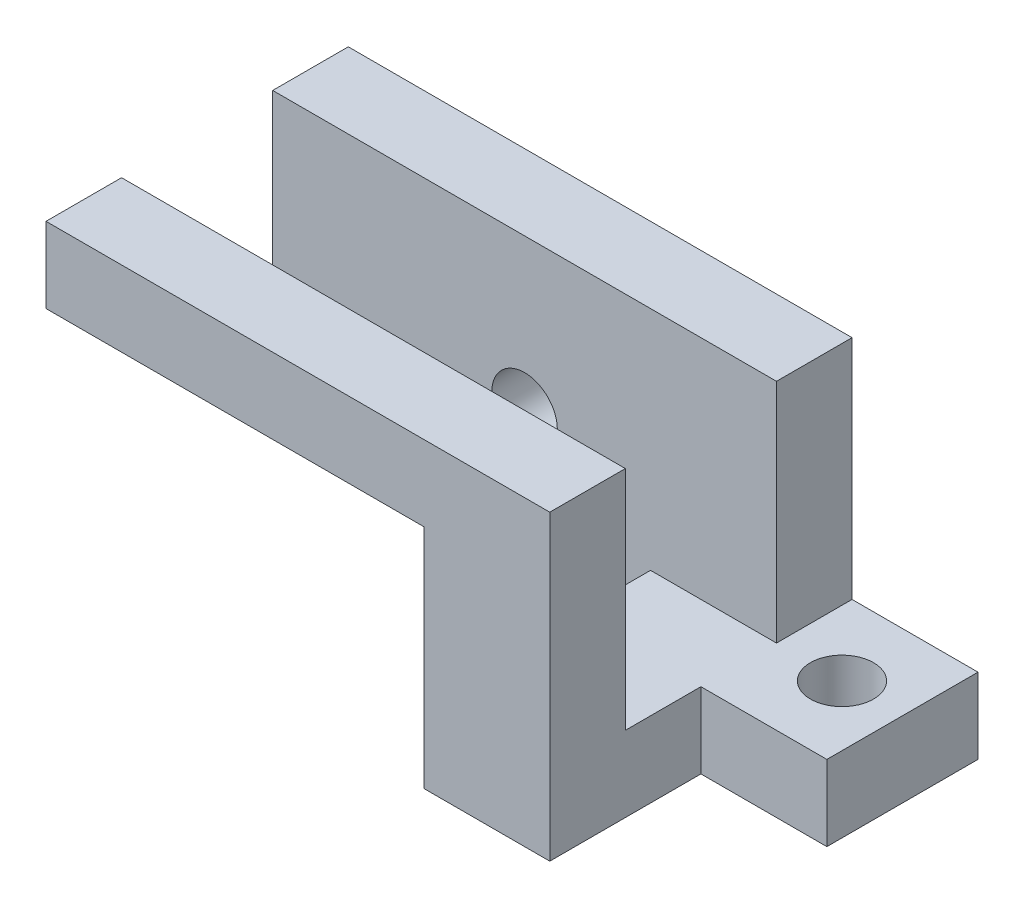
ISO-10303-21;
HEADER;
FILE_DESCRIPTION(('STEP AP214'),'2;1');
FILE_NAME('part.step','',(''),(''),'','','');
FILE_SCHEMA(('AUTOMOTIVE_DESIGN { 1 0 10303 214 1 1 1 1 }'));
ENDSEC;
DATA;
#1=APPLICATION_CONTEXT('core data for automotive mechanical design processes');
#2=APPLICATION_PROTOCOL_DEFINITION('international standard','automotive_design',2000,#1);
#3=PRODUCT_CONTEXT('',#1,'mechanical');
#4=PRODUCT('Part','Part','',(#3));
#5=PRODUCT_RELATED_PRODUCT_CATEGORY('part','',(#4));
#6=PRODUCT_DEFINITION_FORMATION('','',#4);
#7=PRODUCT_DEFINITION_CONTEXT('part definition',#1,'design');
#8=PRODUCT_DEFINITION('design','',#6,#7);
#9=PRODUCT_DEFINITION_SHAPE('','',#8);
#10=(LENGTH_UNIT() NAMED_UNIT(*) SI_UNIT(.MILLI.,.METRE.));
#11=(NAMED_UNIT(*) PLANE_ANGLE_UNIT() SI_UNIT($,.RADIAN.));
#12=(NAMED_UNIT(*) SI_UNIT($,.STERADIAN.) SOLID_ANGLE_UNIT());
#13=UNCERTAINTY_MEASURE_WITH_UNIT(LENGTH_MEASURE(1.E-05),#10,'distance_accuracy_value','');
#14=(GEOMETRIC_REPRESENTATION_CONTEXT(3) GLOBAL_UNCERTAINTY_ASSIGNED_CONTEXT((#13)) GLOBAL_UNIT_ASSIGNED_CONTEXT((#10,
#11,#12)) REPRESENTATION_CONTEXT('',''));
#15=CARTESIAN_POINT('',(0.,0.,0.));
#16=DIRECTION('',(0.,0.,1.));
#17=DIRECTION('',(1.,0.,0.));
#18=AXIS2_PLACEMENT_3D('',#15,#16,#17);
#19=CARTESIAN_POINT('',(0.,-15.,0.));
#20=DIRECTION('',(0.,-1.,0.));
#21=DIRECTION('',(0.,0.,-1.));
#22=AXIS2_PLACEMENT_3D('',#19,#20,#21);
#23=PLANE('',#22);
#24=CARTESIAN_POINT('',(63.,-15.,15.));
#25=DIRECTION('',(0.,-1.,0.));
#26=DIRECTION('',(0.,0.,-1.));
#27=AXIS2_PLACEMENT_3D('',#24,#25,#26);
#28=CIRCLE('',#27,6.26608644715012);
#29=CARTESIAN_POINT('',(63.,-15.,8.73391355284988));
#30=VERTEX_POINT('',#29);
#31=EDGE_CURVE('E192',#30,#30,#28,.T.);
#32=ORIENTED_EDGE('',*,*,#31,.T.);
#33=EDGE_LOOP('',(#32));
#34=FACE_BOUND('',#33,.T.);
#35=DIRECTION('',(-1.,0.,0.));
#36=VECTOR('',#35,1.);
#37=CARTESIAN_POINT('',(0.,-15.,45.));
#38=LINE('',#37,#36);
#39=CARTESIAN_POINT('',(50.,-15.,45.));
#40=VERTEX_POINT('',#39);
#41=CARTESIAN_POINT('',(25.,-15.,45.));
#42=VERTEX_POINT('',#41);
#43=EDGE_CURVE('E184',#40,#42,#38,.T.);
#44=ORIENTED_EDGE('',*,*,#43,.F.);
#45=DIRECTION('',(0.,0.,1.));
#46=VECTOR('',#45,1.);
#47=CARTESIAN_POINT('',(50.,-15.,60.));
#48=LINE('',#47,#46);
#49=CARTESIAN_POINT('',(50.,-15.,30.));
#50=VERTEX_POINT('',#49);
#51=EDGE_CURVE('E146',#50,#40,#48,.T.);
#52=ORIENTED_EDGE('',*,*,#51,.F.);
#53=DIRECTION('',(-1.,0.,0.));
#54=VECTOR('',#53,1.);
#55=CARTESIAN_POINT('',(50.,-15.,30.));
#56=LINE('',#55,#54);
#57=CARTESIAN_POINT('',(75.,-15.,30.));
#58=VERTEX_POINT('',#57);
#59=EDGE_CURVE('E205',#58,#50,#56,.T.);
#60=ORIENTED_EDGE('',*,*,#59,.F.);
#61=DIRECTION('',(0.,0.,1.));
#62=VECTOR('',#61,1.);
#63=CARTESIAN_POINT('',(75.,-15.,30.));
#64=LINE('',#63,#62);
#65=CARTESIAN_POINT('',(75.,-15.,0.));
#66=VERTEX_POINT('',#65);
#67=EDGE_CURVE('E203',#66,#58,#64,.T.);
#68=ORIENTED_EDGE('',*,*,#67,.F.);
#69=DIRECTION('',(1.,0.,0.));
#70=VECTOR('',#69,1.);
#71=CARTESIAN_POINT('',(25.,-15.,0.));
#72=LINE('',#71,#70);
#73=CARTESIAN_POINT('',(50.,-15.,0.));
#74=VERTEX_POINT('',#73);
#75=EDGE_CURVE('E199',#74,#66,#72,.T.);
#76=ORIENTED_EDGE('',*,*,#75,.F.);
#77=DIRECTION('',(0.,0.,1.));
#78=VECTOR('',#77,1.);
#79=CARTESIAN_POINT('',(50.,-15.,15.));
#80=LINE('',#79,#78);
#81=CARTESIAN_POINT('',(50.,-15.,15.));
#82=VERTEX_POINT('',#81);
#83=EDGE_CURVE('E11',#74,#82,#80,.T.);
#84=ORIENTED_EDGE('',*,*,#83,.T.);
#85=DIRECTION('',(-1.,0.,0.));
#86=VECTOR('',#85,1.);
#87=CARTESIAN_POINT('',(0.,-15.,15.));
#88=LINE('',#87,#86);
#89=CARTESIAN_POINT('',(25.,-15.,15.));
#90=VERTEX_POINT('',#89);
#91=EDGE_CURVE('E62',#82,#90,#88,.T.);
#92=ORIENTED_EDGE('',*,*,#91,.T.);
#93=DIRECTION('',(0.,0.,-1.));
#94=VECTOR('',#93,1.);
#95=CARTESIAN_POINT('',(25.,-15.,60.));
#96=LINE('',#95,#94);
#97=EDGE_CURVE('E53',#42,#90,#96,.T.);
#98=ORIENTED_EDGE('',*,*,#97,.F.);
#99=EDGE_LOOP('',(#44,#52,#60,#68,#76,#84,#92,#98));
#100=FACE_BOUND('',#99,.T.);
#101=ADVANCED_FACE('F39',(#34,#100),#23,.F.);
#102=CARTESIAN_POINT('',(50.,-30.,15.));
#103=DIRECTION('',(-1.,0.,0.));
#104=DIRECTION('',(0.,0.,1.));
#105=AXIS2_PLACEMENT_3D('',#102,#103,#104);
#106=PLANE('',#105);
#107=ORIENTED_EDGE('',*,*,#83,.F.);
#108=DIRECTION('',(0.,1.,0.));
#109=VECTOR('',#108,1.);
#110=CARTESIAN_POINT('',(50.,-30.,0.));
#111=LINE('',#110,#109);
#112=CARTESIAN_POINT('',(50.,30.,0.));
#113=VERTEX_POINT('',#112);
#114=EDGE_CURVE('E240',#74,#113,#111,.T.);
#115=ORIENTED_EDGE('',*,*,#114,.T.);
#116=DIRECTION('',(0.,0.,-1.));
#117=VECTOR('',#116,1.);
#118=CARTESIAN_POINT('',(50.,30.,15.));
#119=LINE('',#118,#117);
#120=CARTESIAN_POINT('',(50.,30.,15.));
#121=VERTEX_POINT('',#120);
#122=EDGE_CURVE('E50',#121,#113,#119,.T.);
#123=ORIENTED_EDGE('',*,*,#122,.F.);
#124=DIRECTION('',(0.,1.,0.));
#125=VECTOR('',#124,1.);
#126=CARTESIAN_POINT('',(50.,-30.,15.));
#127=LINE('',#126,#125);
#128=EDGE_CURVE('E239',#82,#121,#127,.T.);
#129=ORIENTED_EDGE('',*,*,#128,.F.);
#130=EDGE_LOOP('',(#107,#115,#123,#129));
#131=FACE_BOUND('',#130,.T.);
#132=ADVANCED_FACE('F41',(#131),#106,.F.);
#133=CARTESIAN_POINT('',(0.,0.,15.));
#134=DIRECTION('',(0.,0.,-1.));
#135=DIRECTION('',(-1.,0.,0.));
#136=AXIS2_PLACEMENT_3D('',#133,#134,#135);
#137=PLANE('',#136);
#138=DIRECTION('',(1.,0.,0.));
#139=VECTOR('',#138,1.);
#140=CARTESIAN_POINT('',(-50.,-30.,15.));
#141=LINE('',#140,#139);
#142=CARTESIAN_POINT('',(-50.,-30.,15.));
#143=VERTEX_POINT('',#142);
#144=CARTESIAN_POINT('',(25.,-30.,15.));
#145=VERTEX_POINT('',#144);
#146=EDGE_CURVE('E250',#143,#145,#141,.T.);
#147=ORIENTED_EDGE('',*,*,#146,.T.);
#148=DIRECTION('',(0.,1.,0.));
#149=VECTOR('',#148,1.);
#150=CARTESIAN_POINT('',(25.,0.,15.));
#151=LINE('',#150,#149);
#152=EDGE_CURVE('E224',#145,#90,#151,.T.);
#153=ORIENTED_EDGE('',*,*,#152,.T.);
#154=ORIENTED_EDGE('',*,*,#91,.F.);
#155=ORIENTED_EDGE('',*,*,#128,.T.);
#156=DIRECTION('',(-1.,0.,0.));
#157=VECTOR('',#156,1.);
#158=CARTESIAN_POINT('',(-50.,30.,15.));
#159=LINE('',#158,#157);
#160=CARTESIAN_POINT('',(-50.,30.,15.));
#161=VERTEX_POINT('',#160);
#162=EDGE_CURVE('E245',#121,#161,#159,.T.);
#163=ORIENTED_EDGE('',*,*,#162,.T.);
#164=DIRECTION('',(0.,-1.,0.));
#165=VECTOR('',#164,1.);
#166=CARTESIAN_POINT('',(-50.,-30.,15.));
#167=LINE('',#166,#165);
#168=EDGE_CURVE('E244',#161,#143,#167,.T.);
#169=ORIENTED_EDGE('',*,*,#168,.T.);
#170=EDGE_LOOP('',(#147,#153,#154,#155,#163,#169));
#171=FACE_BOUND('',#170,.T.);
#172=CARTESIAN_POINT('',(0.,0.,15.));
#173=DIRECTION('',(0.,0.,1.));
#174=DIRECTION('',(1.,0.,0.));
#175=AXIS2_PLACEMENT_3D('',#172,#173,#174);
#176=CIRCLE('',#175,6.5);
#177=CARTESIAN_POINT('',(6.49999999999999,0.,15.));
#178=VERTEX_POINT('',#177);
#179=EDGE_CURVE('E234',#178,#178,#176,.T.);
#180=ORIENTED_EDGE('',*,*,#179,.F.);
#181=EDGE_LOOP('',(#180));
#182=FACE_BOUND('',#181,.T.);
#183=ADVANCED_FACE('F283',(#171,#182),#137,.F.);
#184=CARTESIAN_POINT('',(0.,0.,0.));
#185=DIRECTION('',(0.,0.,-1.));
#186=DIRECTION('',(-1.,0.,0.));
#187=AXIS2_PLACEMENT_3D('',#184,#185,#186);
#188=PLANE('',#187);
#189=DIRECTION('',(0.,-1.,0.));
#190=VECTOR('',#189,1.);
#191=CARTESIAN_POINT('',(75.,-15.,0.));
#192=LINE('',#191,#190);
#193=CARTESIAN_POINT('',(75.,-30.,0.));
#194=VERTEX_POINT('',#193);
#195=EDGE_CURVE('E206',#66,#194,#192,.T.);
#196=ORIENTED_EDGE('',*,*,#195,.T.);
#197=DIRECTION('',(1.,0.,0.));
#198=VECTOR('',#197,1.);
#199=CARTESIAN_POINT('',(-50.,-30.,0.));
#200=LINE('',#199,#198);
#201=CARTESIAN_POINT('',(-50.,-30.,0.));
#202=VERTEX_POINT('',#201);
#203=EDGE_CURVE('E243',#202,#194,#200,.T.);
#204=ORIENTED_EDGE('',*,*,#203,.F.);
#205=DIRECTION('',(0.,-1.,0.));
#206=VECTOR('',#205,1.);
#207=CARTESIAN_POINT('',(-50.,-30.,0.));
#208=LINE('',#207,#206);
#209=CARTESIAN_POINT('',(-50.,30.,0.));
#210=VERTEX_POINT('',#209);
#211=EDGE_CURVE('E251',#210,#202,#208,.T.);
#212=ORIENTED_EDGE('',*,*,#211,.F.);
#213=DIRECTION('',(-1.,0.,0.));
#214=VECTOR('',#213,1.);
#215=CARTESIAN_POINT('',(-50.,30.,0.));
#216=LINE('',#215,#214);
#217=EDGE_CURVE('E255',#113,#210,#216,.T.);
#218=ORIENTED_EDGE('',*,*,#217,.F.);
#219=ORIENTED_EDGE('',*,*,#114,.F.);
#220=ORIENTED_EDGE('',*,*,#75,.T.);
#221=EDGE_LOOP('',(#196,#204,#212,#218,#219,#220));
#222=FACE_BOUND('',#221,.T.);
#223=CARTESIAN_POINT('',(0.,0.,0.));
#224=DIRECTION('',(0.,0.,1.));
#225=DIRECTION('',(1.,0.,0.));
#226=AXIS2_PLACEMENT_3D('',#223,#224,#225);
#227=CIRCLE('',#226,6.5);
#228=CARTESIAN_POINT('',(6.49999999999999,0.,0.));
#229=VERTEX_POINT('',#228);
#230=EDGE_CURVE('E231',#229,#229,#227,.T.);
#231=ORIENTED_EDGE('',*,*,#230,.T.);
#232=EDGE_LOOP('',(#231));
#233=FACE_BOUND('',#232,.T.);
#234=ADVANCED_FACE('F271',(#222,#233),#188,.T.);
#235=CARTESIAN_POINT('',(-50.,30.,15.));
#236=DIRECTION('',(0.,-1.,0.));
#237=DIRECTION('',(0.,0.,-1.));
#238=AXIS2_PLACEMENT_3D('',#235,#236,#237);
#239=PLANE('',#238);
#240=ORIENTED_EDGE('',*,*,#217,.T.);
#241=DIRECTION('',(0.,0.,-1.));
#242=VECTOR('',#241,1.);
#243=CARTESIAN_POINT('',(-50.,30.,15.));
#244=LINE('',#243,#242);
#245=EDGE_CURVE('E256',#161,#210,#244,.T.);
#246=ORIENTED_EDGE('',*,*,#245,.F.);
#247=ORIENTED_EDGE('',*,*,#162,.F.);
#248=ORIENTED_EDGE('',*,*,#122,.T.);
#249=EDGE_LOOP('',(#240,#246,#247,#248));
#250=FACE_BOUND('',#249,.T.);
#251=ADVANCED_FACE('F263',(#250),#239,.F.);
#252=CARTESIAN_POINT('',(-50.,-30.,15.));
#253=DIRECTION('',(1.,0.,0.));
#254=DIRECTION('',(0.,0.,-1.));
#255=AXIS2_PLACEMENT_3D('',#252,#253,#254);
#256=PLANE('',#255);
#257=ORIENTED_EDGE('',*,*,#211,.T.);
#258=DIRECTION('',(0.,0.,-1.));
#259=VECTOR('',#258,1.);
#260=CARTESIAN_POINT('',(-50.,-30.,15.));
#261=LINE('',#260,#259);
#262=EDGE_CURVE('E249',#143,#202,#261,.T.);
#263=ORIENTED_EDGE('',*,*,#262,.F.);
#264=ORIENTED_EDGE('',*,*,#168,.F.);
#265=ORIENTED_EDGE('',*,*,#245,.T.);
#266=EDGE_LOOP('',(#257,#263,#264,#265));
#267=FACE_BOUND('',#266,.T.);
#268=ADVANCED_FACE('F279',(#267),#256,.F.);
#269=CARTESIAN_POINT('',(-50.,-30.,15.));
#270=DIRECTION('',(0.,1.,0.));
#271=DIRECTION('',(0.,0.,1.));
#272=AXIS2_PLACEMENT_3D('',#269,#270,#271);
#273=PLANE('',#272);
#274=DIRECTION('',(0.,0.,-1.));
#275=VECTOR('',#274,1.);
#276=CARTESIAN_POINT('',(25.,-30.,60.));
#277=LINE('',#276,#275);
#278=CARTESIAN_POINT('',(25.,-30.,60.));
#279=VERTEX_POINT('',#278);
#280=EDGE_CURVE('E191',#279,#145,#277,.T.);
#281=ORIENTED_EDGE('',*,*,#280,.T.);
#282=ORIENTED_EDGE('',*,*,#146,.F.);
#283=ORIENTED_EDGE('',*,*,#262,.T.);
#284=ORIENTED_EDGE('',*,*,#203,.T.);
#285=DIRECTION('',(0.,0.,1.));
#286=VECTOR('',#285,1.);
#287=CARTESIAN_POINT('',(75.,-30.,30.));
#288=LINE('',#287,#286);
#289=CARTESIAN_POINT('',(75.,-30.,30.));
#290=VERTEX_POINT('',#289);
#291=EDGE_CURVE('E208',#194,#290,#288,.T.);
#292=ORIENTED_EDGE('',*,*,#291,.T.);
#293=DIRECTION('',(-1.,0.,0.));
#294=VECTOR('',#293,1.);
#295=CARTESIAN_POINT('',(50.,-30.,30.));
#296=LINE('',#295,#294);
#297=CARTESIAN_POINT('',(50.,-30.,30.));
#298=VERTEX_POINT('',#297);
#299=EDGE_CURVE('E214',#290,#298,#296,.T.);
#300=ORIENTED_EDGE('',*,*,#299,.T.);
#301=DIRECTION('',(0.,0.,1.));
#302=VECTOR('',#301,1.);
#303=CARTESIAN_POINT('',(50.,-30.,60.));
#304=LINE('',#303,#302);
#305=CARTESIAN_POINT('',(50.,-30.,60.));
#306=VERTEX_POINT('',#305);
#307=EDGE_CURVE('E217',#298,#306,#304,.T.);
#308=ORIENTED_EDGE('',*,*,#307,.T.);
#309=DIRECTION('',(-1.,0.,0.));
#310=VECTOR('',#309,1.);
#311=CARTESIAN_POINT('',(25.,-30.,60.));
#312=LINE('',#311,#310);
#313=EDGE_CURVE('E196',#306,#279,#312,.T.);
#314=ORIENTED_EDGE('',*,*,#313,.T.);
#315=EDGE_LOOP('',(#281,#282,#283,#284,#292,#300,#308,#314));
#316=FACE_BOUND('',#315,.T.);
#317=CARTESIAN_POINT('',(63.,-30.,15.));
#318=DIRECTION('',(0.,-1.,0.));
#319=DIRECTION('',(0.,0.,-1.));
#320=AXIS2_PLACEMENT_3D('',#317,#318,#319);
#321=CIRCLE('',#320,6.26608644715012);
#322=CARTESIAN_POINT('',(63.,-30.,8.73391355284988));
#323=VERTEX_POINT('',#322);
#324=EDGE_CURVE('E188',#323,#323,#321,.T.);
#325=ORIENTED_EDGE('',*,*,#324,.F.);
#326=EDGE_LOOP('',(#325));
#327=FACE_BOUND('',#326,.T.);
#328=ADVANCED_FACE('F285',(#316,#327),#273,.F.);
#329=CARTESIAN_POINT('',(0.,0.,15.));
#330=DIRECTION('',(0.,0.,-1.));
#331=DIRECTION('',(-1.,0.,0.));
#332=AXIS2_PLACEMENT_3D('',#329,#330,#331);
#333=CYLINDRICAL_SURFACE('',#332,6.5);
#334=ORIENTED_EDGE('',*,*,#179,.T.);
#335=EDGE_LOOP('',(#334));
#336=FACE_BOUND('',#335,.T.);
#337=ORIENTED_EDGE('',*,*,#230,.F.);
#338=EDGE_LOOP('',(#337));
#339=FACE_BOUND('',#338,.T.);
#340=ADVANCED_FACE('F334',(#336,#339),#333,.F.);
#341=CARTESIAN_POINT('',(25.,-15.,60.));
#342=DIRECTION('',(-1.,0.,0.));
#343=DIRECTION('',(0.,0.,1.));
#344=AXIS2_PLACEMENT_3D('',#341,#342,#343);
#345=PLANE('',#344);
#346=DIRECTION('',(0.,-1.,0.));
#347=VECTOR('',#346,1.);
#348=CARTESIAN_POINT('',(25.,-15.,60.));
#349=LINE('',#348,#347);
#350=CARTESIAN_POINT('',(25.,15.,60.));
#351=VERTEX_POINT('',#350);
#352=EDGE_CURVE('E218',#351,#279,#349,.T.);
#353=ORIENTED_EDGE('',*,*,#352,.F.);
#354=DIRECTION('',(0.,0.,1.));
#355=VECTOR('',#354,1.);
#356=CARTESIAN_POINT('',(25.,15.,45.));
#357=LINE('',#356,#355);
#358=CARTESIAN_POINT('',(25.,15.,45.));
#359=VERTEX_POINT('',#358);
#360=EDGE_CURVE('E185',#359,#351,#357,.T.);
#361=ORIENTED_EDGE('',*,*,#360,.F.);
#362=DIRECTION('',(0.,-1.,0.));
#363=VECTOR('',#362,1.);
#364=CARTESIAN_POINT('',(25.,-30.,45.));
#365=LINE('',#364,#363);
#366=EDGE_CURVE('E151',#359,#42,#365,.T.);
#367=ORIENTED_EDGE('',*,*,#366,.T.);
#368=ORIENTED_EDGE('',*,*,#97,.T.);
#369=ORIENTED_EDGE('',*,*,#152,.F.);
#370=ORIENTED_EDGE('',*,*,#280,.F.);
#371=EDGE_LOOP('',(#353,#361,#367,#368,#369,#370));
#372=FACE_BOUND('',#371,.T.);
#373=ADVANCED_FACE('F289',(#372),#345,.T.);
#374=CARTESIAN_POINT('',(25.,-15.,60.));
#375=DIRECTION('',(0.,0.,1.));
#376=DIRECTION('',(1.,0.,0.));
#377=AXIS2_PLACEMENT_3D('',#374,#375,#376);
#378=PLANE('',#377);
#379=ORIENTED_EDGE('',*,*,#313,.F.);
#380=DIRECTION('',(0.,-1.,0.));
#381=VECTOR('',#380,1.);
#382=CARTESIAN_POINT('',(50.,-15.,60.));
#383=LINE('',#382,#381);
#384=CARTESIAN_POINT('',(50.,30.,60.));
#385=VERTEX_POINT('',#384);
#386=EDGE_CURVE('E222',#385,#306,#383,.T.);
#387=ORIENTED_EDGE('',*,*,#386,.F.);
#388=DIRECTION('',(-1.,0.,0.));
#389=VECTOR('',#388,1.);
#390=CARTESIAN_POINT('',(-50.,30.,60.));
#391=LINE('',#390,#389);
#392=CARTESIAN_POINT('',(-50.,30.,60.));
#393=VERTEX_POINT('',#392);
#394=EDGE_CURVE('E156',#385,#393,#391,.T.);
#395=ORIENTED_EDGE('',*,*,#394,.T.);
#396=DIRECTION('',(0.,-1.,0.));
#397=VECTOR('',#396,1.);
#398=CARTESIAN_POINT('',(-50.,30.,60.));
#399=LINE('',#398,#397);
#400=CARTESIAN_POINT('',(-50.,15.,60.));
#401=VERTEX_POINT('',#400);
#402=EDGE_CURVE('E176',#393,#401,#399,.T.);
#403=ORIENTED_EDGE('',*,*,#402,.T.);
#404=DIRECTION('',(1.,0.,0.));
#405=VECTOR('',#404,1.);
#406=CARTESIAN_POINT('',(25.,15.,60.));
#407=LINE('',#406,#405);
#408=EDGE_CURVE('E177',#401,#351,#407,.T.);
#409=ORIENTED_EDGE('',*,*,#408,.T.);
#410=ORIENTED_EDGE('',*,*,#352,.T.);
#411=EDGE_LOOP('',(#379,#387,#395,#403,#409,#410));
#412=FACE_BOUND('',#411,.T.);
#413=ADVANCED_FACE('F293',(#412),#378,.T.);
#414=CARTESIAN_POINT('',(50.,-15.,60.));
#415=DIRECTION('',(1.,0.,0.));
#416=DIRECTION('',(0.,0.,-1.));
#417=AXIS2_PLACEMENT_3D('',#414,#415,#416);
#418=PLANE('',#417);
#419=ORIENTED_EDGE('',*,*,#386,.T.);
#420=ORIENTED_EDGE('',*,*,#307,.F.);
#421=DIRECTION('',(0.,-1.,0.));
#422=VECTOR('',#421,1.);
#423=CARTESIAN_POINT('',(50.,-15.,30.));
#424=LINE('',#423,#422);
#425=EDGE_CURVE('E221',#50,#298,#424,.T.);
#426=ORIENTED_EDGE('',*,*,#425,.F.);
#427=ORIENTED_EDGE('',*,*,#51,.T.);
#428=DIRECTION('',(0.,1.,0.));
#429=VECTOR('',#428,1.);
#430=CARTESIAN_POINT('',(50.,-30.,45.));
#431=LINE('',#430,#429);
#432=CARTESIAN_POINT('',(50.,30.,45.));
#433=VERTEX_POINT('',#432);
#434=EDGE_CURVE('E145',#40,#433,#431,.T.);
#435=ORIENTED_EDGE('',*,*,#434,.T.);
#436=DIRECTION('',(0.,0.,1.));
#437=VECTOR('',#436,1.);
#438=CARTESIAN_POINT('',(50.,30.,45.));
#439=LINE('',#438,#437);
#440=EDGE_CURVE('E147',#433,#385,#439,.T.);
#441=ORIENTED_EDGE('',*,*,#440,.T.);
#442=EDGE_LOOP('',(#419,#420,#426,#427,#435,#441));
#443=FACE_BOUND('',#442,.T.);
#444=ADVANCED_FACE('F143',(#443),#418,.T.);
#445=CARTESIAN_POINT('',(50.,-15.,30.));
#446=DIRECTION('',(0.,0.,1.));
#447=DIRECTION('',(1.,0.,0.));
#448=AXIS2_PLACEMENT_3D('',#445,#446,#447);
#449=PLANE('',#448);
#450=ORIENTED_EDGE('',*,*,#299,.F.);
#451=DIRECTION('',(0.,-1.,0.));
#452=VECTOR('',#451,1.);
#453=CARTESIAN_POINT('',(75.,-15.,30.));
#454=LINE('',#453,#452);
#455=EDGE_CURVE('E227',#58,#290,#454,.T.);
#456=ORIENTED_EDGE('',*,*,#455,.F.);
#457=ORIENTED_EDGE('',*,*,#59,.T.);
#458=ORIENTED_EDGE('',*,*,#425,.T.);
#459=EDGE_LOOP('',(#450,#456,#457,#458));
#460=FACE_BOUND('',#459,.T.);
#461=ADVANCED_FACE('F306',(#460),#449,.T.);
#462=CARTESIAN_POINT('',(75.,-15.,30.));
#463=DIRECTION('',(1.,0.,0.));
#464=DIRECTION('',(0.,0.,-1.));
#465=AXIS2_PLACEMENT_3D('',#462,#463,#464);
#466=PLANE('',#465);
#467=ORIENTED_EDGE('',*,*,#291,.F.);
#468=ORIENTED_EDGE('',*,*,#195,.F.);
#469=ORIENTED_EDGE('',*,*,#67,.T.);
#470=ORIENTED_EDGE('',*,*,#455,.T.);
#471=EDGE_LOOP('',(#467,#468,#469,#470));
#472=FACE_BOUND('',#471,.T.);
#473=ADVANCED_FACE('F303',(#472),#466,.T.);
#474=CARTESIAN_POINT('',(63.,-15.,15.));
#475=DIRECTION('',(0.,-1.,0.));
#476=DIRECTION('',(0.,0.,-1.));
#477=AXIS2_PLACEMENT_3D('',#474,#475,#476);
#478=CYLINDRICAL_SURFACE('',#477,6.26608644715012);
#479=ORIENTED_EDGE('',*,*,#31,.F.);
#480=EDGE_LOOP('',(#479));
#481=FACE_BOUND('',#480,.T.);
#482=ORIENTED_EDGE('',*,*,#324,.T.);
#483=EDGE_LOOP('',(#482));
#484=FACE_BOUND('',#483,.T.);
#485=ADVANCED_FACE('F312',(#481,#484),#478,.F.);
#486=CARTESIAN_POINT('',(0.,0.,45.));
#487=DIRECTION('',(0.,0.,1.));
#488=DIRECTION('',(1.,0.,0.));
#489=AXIS2_PLACEMENT_3D('',#486,#487,#488);
#490=PLANE('',#489);
#491=ORIENTED_EDGE('',*,*,#434,.F.);
#492=ORIENTED_EDGE('',*,*,#43,.T.);
#493=ORIENTED_EDGE('',*,*,#366,.F.);
#494=DIRECTION('',(1.,0.,0.));
#495=VECTOR('',#494,1.);
#496=CARTESIAN_POINT('',(25.,15.,45.));
#497=LINE('',#496,#495);
#498=CARTESIAN_POINT('',(-50.,15.,45.));
#499=VERTEX_POINT('',#498);
#500=EDGE_CURVE('E162',#499,#359,#497,.T.);
#501=ORIENTED_EDGE('',*,*,#500,.F.);
#502=DIRECTION('',(0.,-1.,0.));
#503=VECTOR('',#502,1.);
#504=CARTESIAN_POINT('',(-50.,30.,45.));
#505=LINE('',#504,#503);
#506=CARTESIAN_POINT('',(-50.,30.,45.));
#507=VERTEX_POINT('',#506);
#508=EDGE_CURVE('E166',#507,#499,#505,.T.);
#509=ORIENTED_EDGE('',*,*,#508,.F.);
#510=DIRECTION('',(-1.,0.,0.));
#511=VECTOR('',#510,1.);
#512=CARTESIAN_POINT('',(-50.,30.,45.));
#513=LINE('',#512,#511);
#514=EDGE_CURVE('E154',#433,#507,#513,.T.);
#515=ORIENTED_EDGE('',*,*,#514,.F.);
#516=EDGE_LOOP('',(#491,#492,#493,#501,#509,#515));
#517=FACE_BOUND('',#516,.T.);
#518=ADVANCED_FACE('F164',(#517),#490,.F.);
#519=CARTESIAN_POINT('',(25.,15.,45.));
#520=DIRECTION('',(0.,-1.,0.));
#521=DIRECTION('',(1.,0.,0.));
#522=AXIS2_PLACEMENT_3D('',#519,#520,#521);
#523=PLANE('',#522);
#524=ORIENTED_EDGE('',*,*,#408,.F.);
#525=DIRECTION('',(0.,0.,1.));
#526=VECTOR('',#525,1.);
#527=CARTESIAN_POINT('',(-50.,15.,45.));
#528=LINE('',#527,#526);
#529=EDGE_CURVE('E187',#499,#401,#528,.T.);
#530=ORIENTED_EDGE('',*,*,#529,.F.);
#531=ORIENTED_EDGE('',*,*,#500,.T.);
#532=ORIENTED_EDGE('',*,*,#360,.T.);
#533=EDGE_LOOP('',(#524,#530,#531,#532));
#534=FACE_BOUND('',#533,.T.);
#535=ADVANCED_FACE('F294',(#534),#523,.T.);
#536=CARTESIAN_POINT('',(-50.,30.,45.));
#537=DIRECTION('',(-1.,0.,0.));
#538=DIRECTION('',(0.,-1.,0.));
#539=AXIS2_PLACEMENT_3D('',#536,#537,#538);
#540=PLANE('',#539);
#541=ORIENTED_EDGE('',*,*,#402,.F.);
#542=DIRECTION('',(0.,0.,1.));
#543=VECTOR('',#542,1.);
#544=CARTESIAN_POINT('',(-50.,30.,45.));
#545=LINE('',#544,#543);
#546=EDGE_CURVE('E163',#507,#393,#545,.T.);
#547=ORIENTED_EDGE('',*,*,#546,.F.);
#548=ORIENTED_EDGE('',*,*,#508,.T.);
#549=ORIENTED_EDGE('',*,*,#529,.T.);
#550=EDGE_LOOP('',(#541,#547,#548,#549));
#551=FACE_BOUND('',#550,.T.);
#552=ADVANCED_FACE('F442',(#551),#540,.T.);
#553=CARTESIAN_POINT('',(-50.,30.,45.));
#554=DIRECTION('',(0.,1.,0.));
#555=DIRECTION('',(0.,0.,1.));
#556=AXIS2_PLACEMENT_3D('',#553,#554,#555);
#557=PLANE('',#556);
#558=ORIENTED_EDGE('',*,*,#394,.F.);
#559=ORIENTED_EDGE('',*,*,#440,.F.);
#560=ORIENTED_EDGE('',*,*,#514,.T.);
#561=ORIENTED_EDGE('',*,*,#546,.T.);
#562=EDGE_LOOP('',(#558,#559,#560,#561));
#563=FACE_BOUND('',#562,.T.);
#564=ADVANCED_FACE('F157',(#563),#557,.T.);
#565=CLOSED_SHELL('',(#101,#132,#183,#234,#251,#268,#328,#340,#373,#413,#444,#461,#473,#485,
#518,#535,#552,#564));
#566=MANIFOLD_SOLID_BREP('B2',#565);
#567=ADVANCED_BREP_SHAPE_REPRESENTATION('',(#18,#566),#14);
#568=SHAPE_DEFINITION_REPRESENTATION(#9,#567);
ENDSEC;
END-ISO-10303-21;
